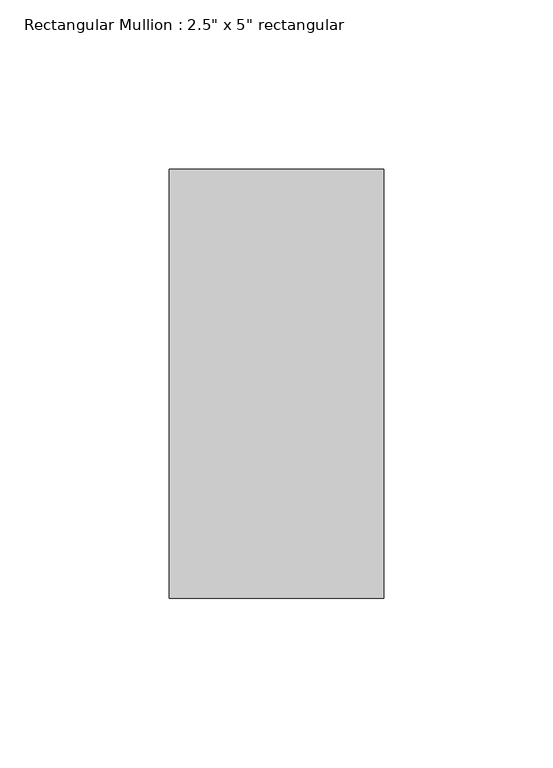
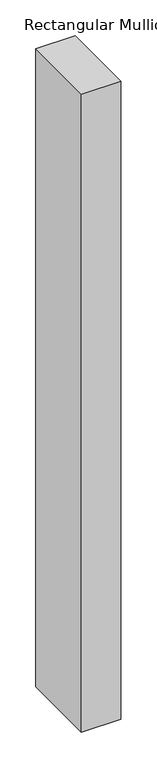
"""IFC4 building model written with IfcOpenShell, lengths in millimetres: member geometry."""

from ifc_helpers import new_model, si_unit, frame, origin, place, context, project, spatial, polyline, outline, extrude, source, transform, mapped, element, save


def member_5474ae84(model_context):
    return source(origin(), model_context, "Body", "SweptSolid", [
        extrude(outline(polyline([(0.0, 63.5), (0.0, -63.5), (-63.5, -63.5), (-63.5, 63.5), (0.0, 63.5)])), frame((0.0, 0.0, -1085.8500002), z_axis=(0.0, 0.0, 1.0), x_axis=(1.0, 0.0, 0.0)), (0.0, 0.0, 1.0), 1085.8500002),
    ])


if __name__ == "__main__":
    model = new_model("IFC4")
    model_context = context("Model", 3, world=origin())
    ifc_project = project(units=[si_unit("LENGTHUNIT", "METRE", prefix="MILLI")], contexts=[model_context])
    site = spatial("IfcSite", under=ifc_project)
    building = spatial("IfcBuilding", under=site)
    placement = place(None, origin())
    member_shape = member_5474ae84(model_context)
    element("IfcMember", 1, ObjectType="Rectangular Mullion : 2.5\" x 5\" rectangular", at=placement, inside=building, context=model_context, shape_type="MappedRepresentation", body=[
        mapped(member_shape, transform((0.0, 0.0, 0.0), x_axis=(1.0, 0.0, 0.0), y_axis=(0.0, 1.0, 0.0), z_axis=(0.0, 0.0, 1.0))),
    ])
    save(model, "model.ifc")

# Revit data of these elements
# Type "Rectangular Mullion : 2.5\" x 5\" rectangular"
#   built-in parameter 1007304 = 0.416667 (stored number, unit not read)
#   built-in parameter 1007301 = 0.104167 (stored number, unit not read)
#   built-in parameter 1007300 = 0.104167 (stored number, unit not read)
# Element 1 (IfcMember, "Rectangular Mullion : 2.5\" x 5\" rectangular")
#   Materials on its faces: "Aluminum"
# Materials
#   "Aluminum": class "Metal", colour RGB 247 247 247, transparency 0, Description = "Aluminum 6061", Cost = 0
